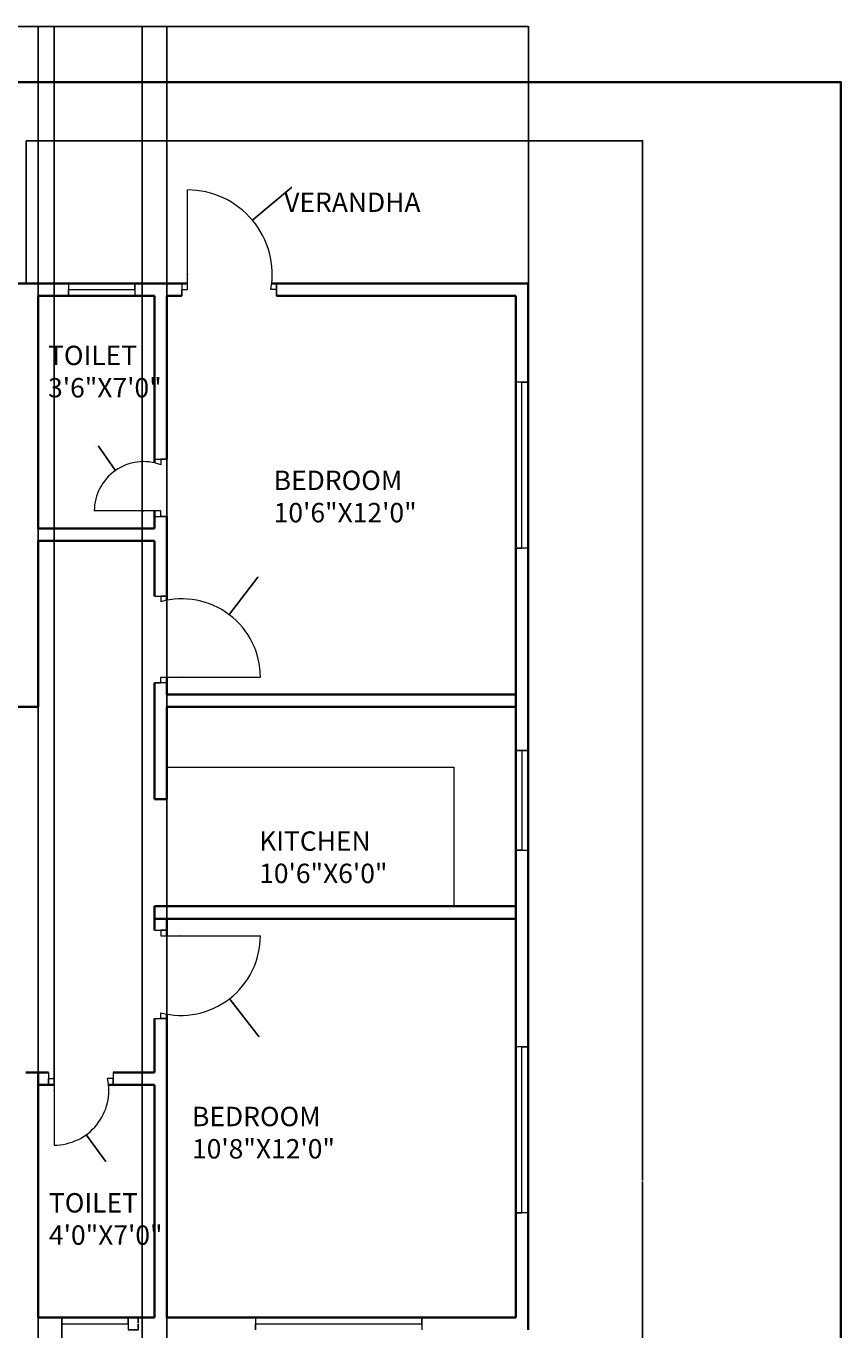
# Model space of a CAD drawing. Units: inches. Extents: x 6393 to 7221, y 6416 to 7347.
# Tile 3 of 3: x 6927 to 7221, y 6876 to 7347. Entities that reach past the tile are written whole.
import ezdxf

# ---------------------------------------------------------------- set-up
doc = ezdxf.new("R2010")
doc.units = ezdxf.units.IN
for name, color, linetype, lineweight in [('A-ANNO-DIMS', 2, 'Continuous', 18), ('A-ANNO-TTLB', 7, 'Continuous', 35), ('A-AREA-IDEN', 7, 'Continuous', 18), ('A-DOOR', 3, 'Continuous', 18), ('A-FLOR-BALC', 7, 'Continuous', 25), ('A-FLOR-FIXT', 8, 'Continuous', 18), ('A-GLAZ', 4, 'Continuous', 18), ('A-WALL', 7, 'Continuous', 35)]:
    doc.layers.add(name, color=color, linetype=linetype, lineweight=lineweight)
doc.styles.get("Standard").update_dxf_attribs({"font": 'arial.ttf'})
doc.dimstyles.get("Standard").update_dxf_attribs({"dimtxt": 0.18, "dimasz": 0.18, "dimexe": 0.18, "dimexo": 0.0625, "dimgap": 0.09, "dimtad": 0, "dimtih": 1, "dimtoh": 1, "dimdec": 4, "dimzin": 0, "dimdsep": 46, "dimtxsty": 'Standard', "dimcen": 0.09, "dimadec": 0, "dimazin": 0, "dimtfac": 1, "dimtdec": 4, "dimtofl": 0, "dimtmove": 0, "dimatfit": 3, "dimfxl": 1, "dimtolj": 1, "dimtzin": 0, "dimarcsym": 0})

# ---------------------------------------------------------------- blocks, each defined once
blk = doc.blocks.new('WIN-60IN')
for p, q in [((0, 60), (4.5, 60)), ((4.5, 60), (2.25, 60)), ((2.25, 60), (2.25, 0)), ((2.25, 0), (0, 0)), ((0, 0), (4.5, 0))]:
    blk.add_line(p, q)
blk = doc.blocks.new('WIN-24IN')
for p, q in [((0, 4.5), (0, 0)), ((0, 0), (0, 2.25)), ((0, 2.25), (24, 2.25)), ((24, 2.25), (24, 4.5)), ((24, 4.5), (24, 0))]:
    blk.add_line(p, q)
blk = doc.blocks.new('VERANDA-EDGE')
for p, q in [((0, 0), (0, 51.5)), ((0, 51.5), (181.5, 51.5)), ((181.5, 51.5), (181.5, 0))]:
    blk.add_line(p, q)
blk = doc.blocks.new('*D8')
at = {"layer": 'A-ANNO-DIMS', "color": 0, "lineweight": -2, "transparency": 16777216}
for p, q in [((6963.97, 6880.83), (6967.68, 6880.83)), ((6967.5, 6880.65), (6967.5, 6878.76)), ((6963.97, 6876.33), (6967.68, 6876.33)), ((6967.5, 6876.51), (6967.5, 6878.4))]:
    blk.add_line(p, q, dxfattribs=at)
at = {"layer": 'A-ANNO-DIMS', "color": 0, "transparency": 16777216}
for points in [[(6967.47, 6880.65), (6967.53, 6880.65), (6967.5, 6880.83)], [(6967.47, 6876.51), (6967.53, 6876.51), (6967.5, 6876.33)]]:
    blk.add_solid(points, dxfattribs=at)
at = {"layer": 'Defpoints', "color": 0, "transparency": 16777216}
for p in [(6963.9, 6880.83), (6967.5, 6880.83), (6963.9, 6876.33)]:
    blk.add_point(p, dxfattribs=at)
at = {"layer": 'A-ANNO-DIMS', "color": 0, "transparency": 16777216, "insert": (6967.5, 6878.58), "char_height": 0.18, "attachment_point": 5}
blk.add_mtext('\\A1;5 TYP.', dxfattribs=at)
blk = doc.blocks.new('*D13')
at = {"layer": 'A-ANNO-DIMS', "color": 0, "lineweight": -2, "transparency": 16777216}
for p, q in [((6476.93, 7305.89), (6476.93, 7347.25)), ((6477.11, 7347.07), (6792.33, 7347.07)), ((7108.35, 7347.07), (6793.12, 7347.07)), ((7108.53, 7305.89), (7108.53, 7347.25))]:
    blk.add_line(p, q, dxfattribs=at)
at = {"layer": 'A-ANNO-DIMS', "color": 0, "transparency": 16777216}
for points in [[(6477.11, 7347.1), (6477.11, 7347.04), (6476.93, 7347.07)], [(7108.35, 7347.1), (7108.35, 7347.04), (7108.53, 7347.07)]]:
    blk.add_solid(points, dxfattribs=at)
at = {"layer": 'Defpoints', "color": 0, "transparency": 16777216}
for p in [(7108.53, 7347.07), (6476.93, 7305.82), (7108.53, 7305.82)]:
    blk.add_point(p, dxfattribs=at)
at = {"layer": 'A-ANNO-DIMS', "color": 0, "transparency": 16777216, "insert": (6792.73, 7347.07), "char_height": 0.18, "attachment_point": 5}
blk.add_mtext('\\A1;631.6', dxfattribs=at)
blk = doc.blocks.new('*D14')
at = {"layer": 'A-ANNO-DIMS', "color": 0, "lineweight": -2, "transparency": 16777216}
for p, q in [((7108.59, 7305.82), (7149.96, 7305.82)), ((7149.78, 7305.64), (7149.78, 6930.26)), ((7149.78, 6554.51), (7149.78, 6929.89)), ((7108.49, 6554.33), (7149.96, 6554.33))]:
    blk.add_line(p, q, dxfattribs=at)
at = {"layer": 'A-ANNO-DIMS', "color": 0, "transparency": 16777216}
for points in [[(7149.75, 7305.64), (7149.81, 7305.64), (7149.78, 7305.82)], [(7149.75, 6554.51), (7149.81, 6554.51), (7149.78, 6554.33)]]:
    blk.add_solid(points, dxfattribs=at)
at = {"layer": 'Defpoints', "color": 0, "transparency": 16777216}
for p in [(7108.53, 7305.82), (7149.78, 7305.82), (7108.43, 6554.33)]:
    blk.add_point(p, dxfattribs=at)
at = {"layer": 'A-ANNO-DIMS', "color": 0, "transparency": 16777216, "insert": (7149.78, 6930.07), "char_height": 0.18, "attachment_point": 5}
blk.add_mtext('\\A1;751.5', dxfattribs=at)
blk = doc.blocks.new('*D29')
at = {"layer": 'A-ANNO-DIMS', "color": 0, "lineweight": -2, "transparency": 16777216}
for p, q in [((6968.93, 6847.89), (6968.93, 7347.25)), ((6969.11, 7347.07), (6973.28, 7347.07)), ((6977.75, 7347.07), (6973.58, 7347.07)), ((6977.93, 6847.89), (6977.93, 7347.25))]:
    blk.add_line(p, q, dxfattribs=at)
at = {"layer": 'A-ANNO-DIMS', "color": 0, "transparency": 16777216}
for points in [[(6969.11, 7347.1), (6969.11, 7347.04), (6968.93, 7347.07)], [(6977.75, 7347.1), (6977.75, 7347.04), (6977.93, 7347.07)]]:
    blk.add_solid(points, dxfattribs=at)
at = {"layer": 'Defpoints', "color": 0, "transparency": 16777216}
for p in [(6977.93, 7347.07), (6968.93, 6847.83), (6977.93, 6847.83)]:
    blk.add_point(p, dxfattribs=at)
at = {"layer": 'A-ANNO-DIMS', "color": 0, "transparency": 16777216, "insert": (6973.43, 7347.07), "char_height": 0.18, "attachment_point": 5}
blk.add_mtext('\\A1;9', dxfattribs=at)
blk = doc.blocks.new('*D32')
at = {"layer": 'A-ANNO-DIMS', "color": 0, "lineweight": -2, "transparency": 16777216}
for p, q in [((6931.43, 6880.76), (6931.43, 6442.29)), ((6939.9, 6880.76), (6939.9, 6442.29)), ((6931.61, 6442.47), (6935.27, 6442.47)), ((6939.72, 6442.47), (6936.06, 6442.47))]:
    blk.add_line(p, q, dxfattribs=at)
at = {"layer": 'A-ANNO-DIMS', "color": 0, "transparency": 16777216}
for points in [[(6931.61, 6442.5), (6931.61, 6442.44), (6931.43, 6442.47)], [(6939.72, 6442.5), (6939.72, 6442.44), (6939.9, 6442.47)]]:
    blk.add_solid(points, dxfattribs=at)
at = {"layer": 'Defpoints', "color": 0, "transparency": 16777216}
for p in [(6931.43, 6880.83), (6939.9, 6880.83), (6939.9, 6442.47)]:
    blk.add_point(p, dxfattribs=at)
at = {"layer": 'A-ANNO-DIMS', "color": 0, "transparency": 16777216, "insert": (6935.67, 6442.47), "char_height": 0.18, "attachment_point": 5}
blk.add_mtext('\\A1;8.477', dxfattribs=at)
blk = doc.blocks.new('*D33')
at = {"layer": 'A-ANNO-DIMS', "color": 0, "lineweight": -2, "transparency": 16777216}
for p, q in [((6931.43, 6964.89), (6931.43, 7347.25)), ((6931.61, 7347.07), (6933.89, 7347.07)), ((6936.96, 7347.07), (6934.68, 7347.07)), ((6937.14, 6964.89), (6937.14, 7347.25))]:
    blk.add_line(p, q, dxfattribs=at)
at = {"layer": 'A-ANNO-DIMS', "color": 0, "transparency": 16777216}
for points in [[(6931.61, 7347.1), (6931.61, 7347.04), (6931.43, 7347.07)], [(6936.96, 7347.1), (6936.96, 7347.04), (6937.14, 7347.07)]]:
    blk.add_solid(points, dxfattribs=at)
at = {"layer": 'Defpoints', "color": 0, "transparency": 16777216}
for p in [(6937.14, 7347.07), (6931.43, 6964.83), (6937.14, 6964.83)]:
    blk.add_point(p, dxfattribs=at)
at = {"layer": 'A-ANNO-DIMS', "color": 0, "transparency": 16777216, "insert": (6934.28, 7347.07), "char_height": 0.18, "attachment_point": 5}
blk.add_mtext('\\A1;5.714', dxfattribs=at)
blk = doc.blocks.new('*D40')
at = {"layer": 'A-ANNO-DIMS', "color": 0, "lineweight": -2, "transparency": 16777216}
for p, q in [((7022.89, 7288.92), (7008.94, 7277.23)), ((7023.07, 7288.92), (7022.89, 7288.92)), ((6985.23, 7257.44), (6985.41, 7257.44)), ((6985.32, 7257.35), (6985.32, 7257.53))]:
    blk.add_line(p, q, dxfattribs=at)
at = {"layer": 'A-ANNO-DIMS', "color": 0, "transparency": 16777216}
blk.add_solid([(7008.92, 7277.25), (7008.96, 7277.21), (7008.8, 7277.12)], dxfattribs=at)
at = {"layer": 'Defpoints', "color": 0, "transparency": 16777216}
for p in [(7008.8, 7277.12), (6985.32, 7257.44)]:
    blk.add_point(p, dxfattribs=at)
at = {"layer": 'A-ANNO-DIMS', "color": 0, "transparency": 16777216, "insert": (7023.62, 7288.92), "char_height": 0.18, "attachment_point": 5}
blk.add_mtext('\\A1;R30.635', dxfattribs=at)
blk = doc.blocks.new('*D44')
at = {"layer": 'A-ANNO-DIMS', "color": 0, "lineweight": -2, "transparency": 16777216}
for p, q in [((6982.81, 7018.7), (6982.99, 7018.7)), ((6982.9, 7018.61), (6982.9, 7018.79)), ((7011.08, 6982.29), (7000.62, 6995.8)), ((7011.26, 6982.29), (7011.08, 6982.29))]:
    blk.add_line(p, q, dxfattribs=at)
at = {"layer": 'A-ANNO-DIMS', "color": 0, "transparency": 16777216}
blk.add_solid([(7000.65, 6995.82), (7000.6, 6995.78), (7000.51, 6995.94)], dxfattribs=at)
at = {"layer": 'Defpoints', "color": 0, "transparency": 16777216}
for p in [(6982.9, 7018.7), (7000.51, 6995.94)]:
    blk.add_point(p, dxfattribs=at)
at = {"layer": 'A-ANNO-DIMS', "color": 0, "transparency": 16777216, "insert": (7011.74, 6982.29), "char_height": 0.18, "attachment_point": 5}
blk.add_mtext('\\A1;R28.78', dxfattribs=at)
blk = doc.blocks.new('*D45')
at = {"layer": 'A-ANNO-DIMS', "color": 0, "lineweight": -2, "transparency": 16777216}
for p, q in [((7010.72, 7148.19), (7000.56, 7134.79)), ((7010.9, 7148.19), (7010.72, 7148.19)), ((6983.25, 7112.06), (6983.43, 7112.06)), ((6983.34, 7111.97), (6983.34, 7112.15))]:
    blk.add_line(p, q, dxfattribs=at)
at = {"layer": 'A-ANNO-DIMS', "color": 0, "transparency": 16777216}
blk.add_solid([(7000.54, 7134.81), (7000.59, 7134.77), (7000.45, 7134.64)], dxfattribs=at)
at = {"layer": 'Defpoints', "color": 0, "transparency": 16777216}
for p in [(7000.45, 7134.64), (6983.34, 7112.06)]:
    blk.add_point(p, dxfattribs=at)
at = {"layer": 'A-ANNO-DIMS', "color": 0, "transparency": 16777216, "insert": (7011.38, 7148.19), "char_height": 0.18, "attachment_point": 5}
blk.add_mtext('\\A1;R28.33', dxfattribs=at)
blk = doc.blocks.new('*D53')
at = {"layer": 'A-ANNO-DIMS', "color": 0, "lineweight": -2, "transparency": 16777216}
for p, q in [((6937.05, 6962.87), (6937.23, 6962.87)), ((6937.14, 6962.78), (6937.14, 6962.96)), ((6955.76, 6937.25), (6948.88, 6946.71)), ((6955.94, 6937.25), (6955.76, 6937.25))]:
    blk.add_line(p, q, dxfattribs=at)
at = {"layer": 'A-ANNO-DIMS', "color": 0, "transparency": 16777216}
blk.add_solid([(6948.91, 6946.73), (6948.86, 6946.69), (6948.78, 6946.86)], dxfattribs=at)
at = {"layer": 'Defpoints', "color": 0, "transparency": 16777216}
for p in [(6937.14, 6962.87), (6948.78, 6946.86)]:
    blk.add_point(p, dxfattribs=at)
at = {"layer": 'A-ANNO-DIMS', "color": 0, "transparency": 16777216, "insert": (6956.49, 6937.25), "char_height": 0.18, "attachment_point": 5}
blk.add_mtext('\\A1;R19.797', dxfattribs=at)
blk = doc.blocks.new('*D55')
at = {"layer": 'A-ANNO-DIMS', "color": 0, "lineweight": -2, "transparency": 16777216}
for p, q in [((6953.04, 7195.52), (6953.22, 7195.52)), ((6953.22, 7195.52), (6959.21, 7186.89)), ((6969.48, 7172.04), (6969.48, 7172.22)), ((6969.39, 7172.13), (6969.57, 7172.13))]:
    blk.add_line(p, q, dxfattribs=at)
at = {"layer": 'A-ANNO-DIMS', "color": 0, "transparency": 16777216}
blk.add_solid([(6959.24, 7186.91), (6959.19, 7186.88), (6959.32, 7186.75)], dxfattribs=at)
at = {"layer": 'Defpoints', "color": 0, "transparency": 16777216}
for p in [(6959.32, 7186.75), (6969.48, 7172.13)]:
    blk.add_point(p, dxfattribs=at)
at = {"layer": 'A-ANNO-DIMS', "color": 0, "transparency": 16777216, "insert": (6952.49, 7195.52), "char_height": 0.18, "attachment_point": 5}
blk.add_mtext('\\A1;R17.802', dxfattribs=at)

msp = doc.modelspace()

# ---------------------------------------------------------------- linework, layer by layer
at = {"layer": 'A-ANNO-TTLB'}
msp.add_lwpolyline([(6392.5039, 7327.0003), (7221.4173, 7327.0003), (7221.4173, 6416.0496), (6392.5039, 6416.0496)], close=True, dxfattribs=at)
at = {"layer": 'A-DOOR'}
for p, q in [((6985.3208, 7252.0767), (6985.3208, 7288.0767)), ((6983.3208, 7254.3267), (6983.3208, 7249.8267)), ((7017.4821, 7254.3267), (7017.4821, 7249.8267)), ((7017.4821, 7249.8267), (7017.4821, 7254.3267)), ((7017.4821, 7254.3267), (7017.4821, 7252.0767)), ((6983.3208, 7249.8267), (6983.3208, 7252.0767)), ((6983.3208, 7252.0767), (6985.3208, 7252.0767)), ((7017.4821, 7252.0767), (7015.4821, 7252.0767)), ((6973.4273, 7190.8178), (6977.9273, 7190.8178)), ((6977.9273, 7190.8178), (6975.6773, 7190.8178)), ((6975.6773, 7190.8178), (6975.6773, 7188.8178)), ((6975.6773, 7172.1297), (6951.6773, 7172.1297)), ((6973.4273, 7170.1297), (6977.9273, 7170.1297)), ((6975.6773, 7170.1297), (6975.6773, 7172.1297)), ((6977.9273, 7170.1297), (6975.6773, 7170.1297)), ((6973.4273, 7141.3364), (6977.9273, 7141.3364)), ((6977.9273, 7141.3364), (6975.6773, 7141.3364)), ((6975.6773, 7141.3364), (6975.6773, 7139.3364)), ((6975.6773, 7110.0609), (6975.6773, 7112.0609)), ((6975.6773, 7112.0609), (7011.6773, 7112.0609)), ((6977.9273, 7110.0609), (6973.4273, 7110.0609)), ((6973.4273, 7110.0609), (6975.6773, 7110.0609)), ((6973.4273, 7020.7027), (6977.9273, 7020.7027)), ((6977.9273, 7020.7027), (6975.6773, 7020.7027)), ((6975.6773, 7020.7027), (6975.6773, 7018.7027)), ((6975.6773, 7018.7027), (7011.6773, 7018.7027)), ((6973.4273, 6988.8444), (6977.9273, 6988.8444)), ((6975.6773, 6988.8444), (6975.6773, 6990.8444)), ((6977.9273, 6988.8444), (6975.6773, 6988.8444)), ((6935.1409, 6969.3267), (6935.1409, 6964.8267)), ((6935.1409, 6964.8267), (6935.1409, 6967.0767)), ((6935.1409, 6967.0767), (6937.1409, 6967.0767)), ((6937.1409, 6967.0767), (6937.1409, 6943.0767)), ((6958.4867, 6967.0767), (6956.4867, 6967.0767)), ((6958.4867, 6969.3267), (6958.4867, 6964.8267)), ((6958.4867, 6964.8267), (6958.4867, 6967.0767))]:
    msp.add_line(p, q, dxfattribs=at)
for centre, radius, start, end in [((6985.3208, 7257.442), 30.6347, 349.91337, 90), ((6969.4792, 7172.1297), 17.8019, 69.624676, 180), ((6983.3445, 7112.0609), 28.3327, 360, 105.700875), ((6982.8983, 7018.7027), 28.7789, 255.468359, 360), ((6937.1409, 6962.8738), 19.7971, 270, 12.25718)]:
    msp.add_arc(centre, radius, start, end, dxfattribs=at)
at = {"layer": 'A-FLOR-FIXT'}
for p, q in [((6977.9273, 7079.5487), (7081.5534, 7079.5487)), ((7081.5534, 7079.5487), (7081.5534, 7029.3267))]:
    msp.add_line(p, q, dxfattribs=at)
at = {"layer": 'A-GLAZ'}
for p, q in [((7103.9273, 7085.5761), (7108.4273, 7085.5761)), ((7108.4273, 7085.5761), (7103.9273, 7085.5761)), ((7106.1773, 7085.5761), (7106.1773, 7049.5761)), ((7106.1773, 7049.5761), (7103.9273, 7049.5761)), ((7103.9273, 7049.5761), (7108.4273, 7049.5761))]:
    msp.add_line(p, q, dxfattribs=at)
at = {"layer": 'A-WALL'}
for p, q in [((6597.6967, 7254.3267), (6985.3208, 7254.3267)), ((6597.6967, 7254.3267), (6985.3208, 7254.3267)), ((7015.7967, 7254.3267), (7108.4273, 7254.3267)), ((7015.7967, 7254.3267), (7108.4273, 7254.3267)), ((7108.4273, 7254.3267), (7108.4273, 6876.3267)), ((6931.4273, 7249.8267), (6931.4273, 7165.8267)), ((6931.4273, 7249.8267), (6973.4273, 7249.8267)), ((6973.4273, 7249.8267), (6973.4273, 7189.4883)), ((6977.9273, 7249.8267), (6977.9273, 7190.8178)), ((6977.9273, 7249.8267), (6983.3208, 7249.8267)), ((7017.4821, 7249.8267), (7103.9273, 7249.8267)), ((7103.9273, 7249.8267), (7103.9273, 6880.8267)), ((6973.4273, 7172.1297), (6973.4273, 7165.8267)), ((6977.9273, 7170.1297), (6977.9273, 7139.8709)), ((6931.4273, 7165.8267), (6973.4273, 7165.8267)), ((6931.4273, 7161.3267), (6973.4273, 7161.3267)), ((6931.4273, 7161.3267), (6931.4273, 7101.3267)), ((6973.4273, 7161.3267), (6973.4273, 7141.3364)), ((6977.9273, 7112.0609), (6977.9273, 7105.8267)), ((6973.4273, 7110.0609), (6973.4273, 7067.9769)), ((6977.9273, 7105.8267), (7103.9273, 7105.8267)), ((6918.6614, 7101.3267), (6931.4273, 7101.3267)), ((6977.9273, 7101.3267), (7103.9273, 7101.3267)), ((6977.9273, 7101.3267), (6977.9273, 7067.9769)), ((6977.9273, 7067.9769), (6973.4273, 7067.9769)), ((6973.4273, 7029.3267), (7103.9273, 7029.3267)), ((6973.4273, 7029.3267), (6973.4273, 7020.7027)), ((6973.4273, 7024.8267), (7103.9273, 7024.8267)), ((6977.9273, 7024.8267), (6977.9273, 7018.7027)), ((6973.4273, 6988.8444), (6973.4273, 6969.3267)), ((6977.9273, 6990.3563), (6977.9273, 6880.8267)), ((6935.1409, 6969.3267), (6926.9273, 6969.3267)), ((6931.4273, 6969.3267), (6931.4273, 6880.8267)), ((6973.4273, 6969.3267), (6958.4867, 6969.3267)), ((6931.4273, 6880.8267), (6931.4273, 6964.8267)), ((6931.4273, 6964.8267), (6937.1409, 6964.8267)), ((6956.8415, 6964.8267), (6973.4273, 6964.8267)), ((6973.4273, 6964.8267), (6973.4273, 6880.8267)), ((6931.4273, 6880.8267), (6973.4273, 6880.8267)), ((6977.9273, 6880.8267), (7103.9273, 6880.8267))]:
    msp.add_line(p, q, dxfattribs=at)

# ---------------------------------------------------------------- block references
at = {"layer": 'A-FLOR-BALC'}
msp.add_blockref('VERANDA-EDGE', (6927.0271, 7254.327), dxfattribs=at)
at = {"layer": 'A-GLAZ'}
for p in [(6942.3801, 7249.827), (6939.905, 6876.327)]:
    msp.add_blockref('WIN-24IN', p, dxfattribs=at)
at = {"layer": 'A-GLAZ', "rotation": 180}
for p in [(7108.4275, 7218.6544), (7108.4275, 6978.5599)]:
    msp.add_blockref('WIN-60IN', p, dxfattribs=at)
at = {"layer": 'A-GLAZ', "extrusion": (0, 0, -1), "zscale": -1, "rotation": 270}
msp.add_blockref('WIN-60IN', (-7069.9641, 6880.827), dxfattribs=at)

# ---------------------------------------------------------------- texts
at = {"layer": 'A-AREA-IDEN', "char_height": 7, "attachment_point": 1}
for s, width, insert in [('VERANDHA', 116.976107, (7020.3044, 7287.126)), ('TOILET\\P3\'6"X7\'0"', 63.559092, (6934.9744, 7231.7945)), ('BEDROOM\\P10\'6"X12\'0"', 108.688083, (7016.4917, 7186.6861)), ('KITCHEN\\P10\'6"X6\'0"', 57.371514, (7011.2475, 7056.3835)), ('BEDROOM\\P10\'8"X12\'0"', 93.30085, (6986.9873, 6956.9115)), ('TOILET\\P4\'0"X7\'0"', 35.997955, (6935.2992, 6925.7362))]:
    msp.add_mtext_dynamic_manual_height_columns(s, width=width, gutter_width=12.5, heights=[0], dxfattribs=dict(at, insert=insert))

# ---------------------------------------------------------------- dimensions: what is measured, and where the dimension line sits
at = {"layer": 'A-ANNO-DIMS'}
for base, p1, p2, override, picture, middle in [((7108.5274, 7347.0726), (6476.9273, 7305.8226), (7108.5274, 7305.8226), {"dimdec": 1, "dimlfac": 1, "dimrnd": 0, "dimzin": 0, "dimdsep": 46, "dimlunit": 2}, '*D13', (6792.7273, 7347.0726)), ((6937.1409, 7347.0726), (6931.4273, 6964.8267), (6937.1409, 6964.8267), {"dimdec": 3, "dimlfac": 1, "dimrnd": 0, "dimzin": 0, "dimdsep": 46, "dimlunit": 2}, '*D33', (6934.2841, 7347.0726)), ((6977.9273, 7347.0726), (6968.9273, 6847.8267), (6977.9273, 6847.8267), {"dimdec": 0, "dimlfac": 1, "dimrnd": 0, "dimzin": 0, "dimdsep": 46, "dimlunit": 2}, '*D29', (6973.4273, 7347.0726)), ((6939.9047, 6442.4706), (6931.4273, 6880.8267), (6939.9047, 6880.8267), {"dimdec": 3, "dimlfac": 1, "dimrnd": 0, "dimzin": 0, "dimdsep": 46, "dimlunit": 2}, '*D32', (6935.666, 6442.4706))]:
    dim = msp.add_linear_dim(base=base, p1=p1, p2=p2, dimstyle='Standard', override=override, dxfattribs=at)
    dim.commit()
    dim.dimension.update_dxf_attribs({"geometry": picture, "text_midpoint": middle})
dim = msp.add_linear_dim(base=(7149.7774, 7305.8226), p1=(7108.4273, 6554.3267), p2=(7108.5274, 7305.8226), angle=90, dimstyle='Standard', override={"dimdec": 1, "dimlfac": 1, "dimrnd": 0, "dimzin": 0, "dimdsep": 46, "dimlunit": 2}, dxfattribs=at)
dim.commit()
dim.dimension.update_dxf_attribs({"geometry": '*D14', "text_midpoint": (7149.7774, 6930.0747)})
for center, mpoint, override, picture, middle in [((6985.3208, 7257.442), (7008.8031, 7277.1161), {"dimdec": 3, "dimlfac": 1, "dimrnd": 0, "dimzin": 0, "dimdsep": 46, "dimlunit": 2}, '*D40', (7023.6229, 7288.9205)), ((6969.4792, 7172.1297), (6959.3163, 7186.7456), {"dimdec": 3, "dimlfac": 1, "dimrnd": 0, "dimzin": 0, "dimdsep": 46, "dimlunit": 2}, '*D55', (6952.4897, 7195.5151)), ((6983.3445, 7112.0609), (7000.4548, 7134.6437), {"dimdec": 2, "dimlfac": 1, "dimrnd": 0, "dimzin": 0, "dimdsep": 46, "dimlunit": 2}, '*D45', (7011.3807, 7148.1934)), ((6982.8983, 7018.7027), (7000.5112, 6995.9428), {"dimdec": 2, "dimlfac": 1, "dimrnd": 0, "dimzin": 0, "dimdsep": 46, "dimlunit": 2}, '*D44', (7011.7389, 6982.2868)), ((6937.1409, 6962.8738), (6948.7768, 6946.8572), {"dimdec": 3, "dimlfac": 1, "dimrnd": 0, "dimzin": 0, "dimdsep": 46, "dimlunit": 2}, '*D53', (6956.4881, 6937.2473))]:
    dim = msp.add_radius_dim(center=center, mpoint=mpoint, dimstyle='Standard', override=override, dxfattribs=at)
    dim.commit()
    dim.dimension.update_dxf_attribs({"geometry": picture, "text_midpoint": middle, "dimtype": 164})
dim = msp.add_linear_dim(base=(6967.5047315606, 6880.8267298921), p1=(6963.9047315606, 6876.3267298921), p2=(6963.9047315606, 6880.8267298921), angle=90, text='<> TYP.', dimstyle='Standard', override={"dimdec": 0, "dimlfac": 1, "dimrnd": 0, "dimzin": 0, "dimdsep": 46, "dimlunit": 2}, dxfattribs=at)
dim.commit()
dim.dimension.update_dxf_attribs({"geometry": '*D8', "text_midpoint": (6967.5047315606, 6878.5767298921)})

doc.saveas('drawing.dxf')
